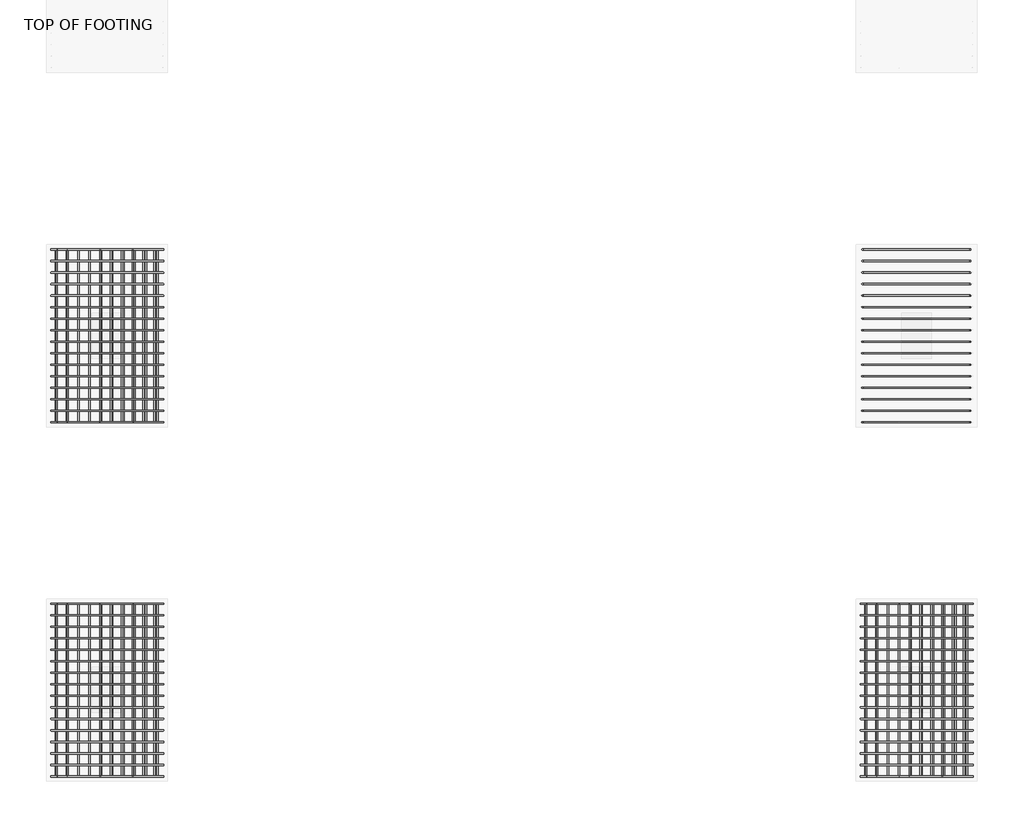
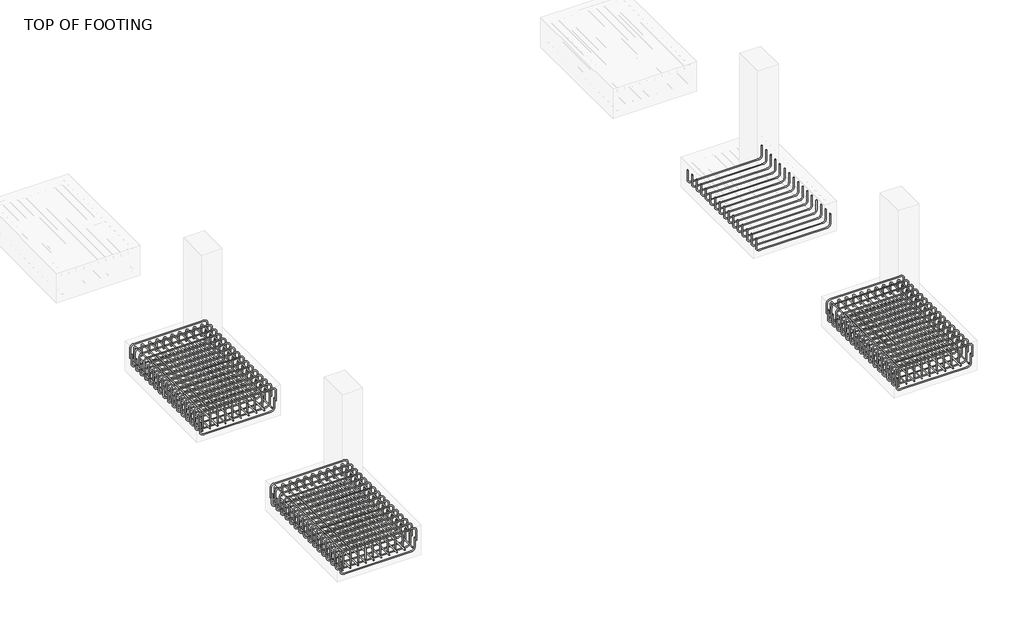
# One storey, part 2 of 8: 13 reinforcing bars.
"""IFC4 building model written with IfcOpenShell, lengths in millimetres."""

from ifc_helpers import new_model, si_unit, point, frame, origin, place, context, project, spatial, polyline, circle_curve, trimmed, segment, composite_curve, source, transform, mapped, element, save
from ifc_brep_helpers import swept_disk

model = new_model("IFC4")

# Units and contexts
model_context = context("Model", 3, world=origin())
ifc_project = project(units=[si_unit("LENGTHUNIT", "METRE", prefix="MILLI")], contexts=[model_context])

# Site, building, storey
site = spatial("IfcSite", under=ifc_project)
building = spatial("IfcBuilding", under=site)
storey = spatial("IfcBuildingStorey", under=building, Name="TOP OF FOOTING", Elevation=-1828.8)

# Reinforcing bars
placement = place(None, origin())
reinforcing_bar_shape = source(origin(), model_context, "Body", "SolidModel", [
    swept_disk(composite_curve([segment(polyline([(-11301.5220197, 6126.3508557, -2021.4413313), (-11301.5220197, 6126.3508557, -2168.7413313)]), True, "CONTINUOUS"), segment(trimmed(circle_curve(frame((-11347.8720197, 6126.3508557, -2168.7413313), z_axis=(0.0, 1.0, 0.0), x_axis=(46.350000000000364, 0.0, 0.0)), 46.35), [point((-11301.5220197, 6126.3508557, -2168.7413313))], [point((-11347.8720197, 6126.3508557, -2215.0913313))], True, "CARTESIAN"), True, "CONTINUOUS"), segment(polyline([(-11347.8720197, 6126.3508557, -2215.0913313), (-12320.167031, 6126.3508557, -2215.0913313)]), True, "CONTINUOUS"), segment(trimmed(circle_curve(frame((-12320.167031, 6126.3508557, -2168.7413313), z_axis=(0.0, 1.0, 0.0), x_axis=(0.0, 0.0, -46.34999999999991)), 46.35), [point((-12320.167031, 6126.3508557, -2215.0913313))], [point((-12366.517031, 6126.3508557, -2168.7413313))], True, "CARTESIAN"), True, "CONTINUOUS"), segment(polyline([(-12366.517031, 6126.3508557, -2168.7413313), (-12366.517031, 6126.3508557, -2021.4413313)]), True, "CONTINUOUS")], self_intersect=False), 6.35),
])
element("IfcReinforcingBar", 1, at=placement, inside=storey, context=model_context, shape_type="MappedRepresentation", body=[
    mapped(reinforcing_bar_shape, transform((0.0, 0.0, 0.0), x_axis=(1.0, 0.0, 0.0), y_axis=(0.0, 1.0, 0.0), z_axis=(0.0, 0.0, 1.0))),
    mapped(reinforcing_bar_shape, transform((0.0, -113.82, 0.0), x_axis=(1.0, 0.0, 0.0), y_axis=(0.0, 1.0, 0.0), z_axis=(0.0, 0.0, 1.0))),
    mapped(reinforcing_bar_shape, transform((0.0, -227.64, 0.0), x_axis=(1.0, 0.0, 0.0), y_axis=(0.0, 1.0, 0.0), z_axis=(0.0, 0.0, 1.0))),
    mapped(reinforcing_bar_shape, transform((0.0, -341.46, 0.0), x_axis=(1.0, 0.0, 0.0), y_axis=(0.0, 1.0, 0.0), z_axis=(0.0, 0.0, 1.0))),
    mapped(reinforcing_bar_shape, transform((0.0, -455.28, 0.0), x_axis=(1.0, 0.0, 0.0), y_axis=(0.0, 1.0, 0.0), z_axis=(0.0, 0.0, 1.0))),
    mapped(reinforcing_bar_shape, transform((0.0, -569.1, 0.0), x_axis=(1.0, 0.0, 0.0), y_axis=(0.0, 1.0, 0.0), z_axis=(0.0, 0.0, 1.0))),
    mapped(reinforcing_bar_shape, transform((0.0, -682.92, 0.0), x_axis=(1.0, 0.0, 0.0), y_axis=(0.0, 1.0, 0.0), z_axis=(0.0, 0.0, 1.0))),
    mapped(reinforcing_bar_shape, transform((0.0, -796.74, 0.0), x_axis=(1.0, 0.0, 0.0), y_axis=(0.0, 1.0, 0.0), z_axis=(0.0, 0.0, 1.0))),
    mapped(reinforcing_bar_shape, transform((0.0, -910.56, 0.0), x_axis=(1.0, 0.0, 0.0), y_axis=(0.0, 1.0, 0.0), z_axis=(0.0, 0.0, 1.0))),
    mapped(reinforcing_bar_shape, transform((0.0, -1024.38, 0.0), x_axis=(1.0, 0.0, 0.0), y_axis=(0.0, 1.0, 0.0), z_axis=(0.0, 0.0, 1.0))),
    mapped(reinforcing_bar_shape, transform((0.0, -1138.2, 0.0), x_axis=(1.0, 0.0, 0.0), y_axis=(0.0, 1.0, 0.0), z_axis=(0.0, 0.0, 1.0))),
    mapped(reinforcing_bar_shape, transform((0.0, -1252.02, 0.0), x_axis=(1.0, 0.0, 0.0), y_axis=(0.0, 1.0, 0.0), z_axis=(0.0, 0.0, 1.0))),
    mapped(reinforcing_bar_shape, transform((0.0, -1365.84, 0.0), x_axis=(1.0, 0.0, 0.0), y_axis=(0.0, 1.0, 0.0), z_axis=(0.0, 0.0, 1.0))),
    mapped(reinforcing_bar_shape, transform((0.0, -1479.66, 0.0), x_axis=(1.0, 0.0, 0.0), y_axis=(0.0, 1.0, 0.0), z_axis=(0.0, 0.0, 1.0))),
    mapped(reinforcing_bar_shape, transform((0.0, -1593.48, 0.0), x_axis=(1.0, 0.0, 0.0), y_axis=(0.0, 1.0, 0.0), z_axis=(0.0, 0.0, 1.0))),
    mapped(reinforcing_bar_shape, transform((0.0, -1707.3, 0.0), x_axis=(1.0, 0.0, 0.0), y_axis=(0.0, 1.0, 0.0), z_axis=(0.0, 0.0, 1.0))),
])
reinforcing_bar_2_shape = source(origin(), model_context, "Body", "SolidModel", [
    swept_disk(composite_curve([segment(polyline([(-12384.3374017, 6126.3508557, -2068.8), (-12384.3374017, 6126.3508557, -1921.5)]), True, "CONTINUOUS"), segment(trimmed(circle_curve(frame((-12337.9874017, 6126.3508557, -1921.5), z_axis=(0.0, 1.0, 0.0), x_axis=(-46.350000000000364, 0.0, 0.0)), 46.35), [point((-12384.3374017, 6126.3508557, -1921.5))], [point((-12337.9874017, 6126.3508557, -1875.15))], True, "CARTESIAN"), True, "CONTINUOUS"), segment(polyline([(-12337.9874017, 6126.3508557, -1875.15), (-11323.3874017, 6126.3508557, -1875.15)]), True, "CONTINUOUS"), segment(trimmed(circle_curve(frame((-11323.3874017, 6126.3508557, -1921.5), z_axis=(0.0, 1.0, 0.0), x_axis=(0.0, 0.0, 46.34999999999991)), 46.35), [point((-11323.3874017, 6126.3508557, -1875.15))], [point((-11277.0374017, 6126.3508557, -1921.5))], True, "CARTESIAN"), True, "CONTINUOUS"), segment(polyline([(-11277.0374017, 6126.3508557, -1921.5), (-11277.0374017, 6126.3508557, -2068.8)]), True, "CONTINUOUS")], self_intersect=False), 6.35),
])
element("IfcReinforcingBar", 2, at=placement, inside=storey, context=model_context, shape_type="MappedRepresentation", body=[
    mapped(reinforcing_bar_2_shape, transform((0.0, 0.0, 0.0), x_axis=(1.0, 0.0, 0.0), y_axis=(0.0, 1.0, 0.0), z_axis=(0.0, 0.0, 1.0))),
    mapped(reinforcing_bar_2_shape, transform((0.0, -113.82, 0.0), x_axis=(1.0, 0.0, 0.0), y_axis=(0.0, 1.0, 0.0), z_axis=(0.0, 0.0, 1.0))),
    mapped(reinforcing_bar_2_shape, transform((0.0, -227.64, 0.0), x_axis=(1.0, 0.0, 0.0), y_axis=(0.0, 1.0, 0.0), z_axis=(0.0, 0.0, 1.0))),
    mapped(reinforcing_bar_2_shape, transform((0.0, -341.46, 0.0), x_axis=(1.0, 0.0, 0.0), y_axis=(0.0, 1.0, 0.0), z_axis=(0.0, 0.0, 1.0))),
    mapped(reinforcing_bar_2_shape, transform((0.0, -455.28, 0.0), x_axis=(1.0, 0.0, 0.0), y_axis=(0.0, 1.0, 0.0), z_axis=(0.0, 0.0, 1.0))),
    mapped(reinforcing_bar_2_shape, transform((0.0, -569.1, 0.0), x_axis=(1.0, 0.0, 0.0), y_axis=(0.0, 1.0, 0.0), z_axis=(0.0, 0.0, 1.0))),
    mapped(reinforcing_bar_2_shape, transform((0.0, -682.92, 0.0), x_axis=(1.0, 0.0, 0.0), y_axis=(0.0, 1.0, 0.0), z_axis=(0.0, 0.0, 1.0))),
    mapped(reinforcing_bar_2_shape, transform((0.0, -796.74, 0.0), x_axis=(1.0, 0.0, 0.0), y_axis=(0.0, 1.0, 0.0), z_axis=(0.0, 0.0, 1.0))),
    mapped(reinforcing_bar_2_shape, transform((0.0, -910.56, 0.0), x_axis=(1.0, 0.0, 0.0), y_axis=(0.0, 1.0, 0.0), z_axis=(0.0, 0.0, 1.0))),
    mapped(reinforcing_bar_2_shape, transform((0.0, -1024.38, 0.0), x_axis=(1.0, 0.0, 0.0), y_axis=(0.0, 1.0, 0.0), z_axis=(0.0, 0.0, 1.0))),
    mapped(reinforcing_bar_2_shape, transform((0.0, -1138.2, 0.0), x_axis=(1.0, 0.0, 0.0), y_axis=(0.0, 1.0, 0.0), z_axis=(0.0, 0.0, 1.0))),
    mapped(reinforcing_bar_2_shape, transform((0.0, -1252.02, 0.0), x_axis=(1.0, 0.0, 0.0), y_axis=(0.0, 1.0, 0.0), z_axis=(0.0, 0.0, 1.0))),
    mapped(reinforcing_bar_2_shape, transform((0.0, -1365.84, 0.0), x_axis=(1.0, 0.0, 0.0), y_axis=(0.0, 1.0, 0.0), z_axis=(0.0, 0.0, 1.0))),
    mapped(reinforcing_bar_2_shape, transform((0.0, -1479.66, 0.0), x_axis=(1.0, 0.0, 0.0), y_axis=(0.0, 1.0, 0.0), z_axis=(0.0, 0.0, 1.0))),
    mapped(reinforcing_bar_2_shape, transform((0.0, -1593.48, 0.0), x_axis=(1.0, 0.0, 0.0), y_axis=(0.0, 1.0, 0.0), z_axis=(0.0, 0.0, 1.0))),
    mapped(reinforcing_bar_2_shape, transform((0.0, -1707.3, 0.0), x_axis=(1.0, 0.0, 0.0), y_axis=(0.0, 1.0, 0.0), z_axis=(0.0, 0.0, 1.0))),
])
reinforcing_bar_3_shape = source(origin(), model_context, "Body", "SolidModel", [
    swept_disk(composite_curve([segment(polyline([(-12339.592709, 6132.7008557, -2155.1176129), (-12339.592709, 4412.7008557, -2155.1176129)]), True, "CONTINUOUS")], self_intersect=False), 6.35),
])
element("IfcReinforcingBar", 3, at=placement, inside=storey, context=model_context, shape_type="MappedRepresentation", body=[
    mapped(reinforcing_bar_3_shape, transform((0.0, 0.0, 0.0), x_axis=(1.0, 0.0, 0.0), y_axis=(0.0, 1.0, 0.0), z_axis=(0.0, 0.0, 1.0))),
    mapped(reinforcing_bar_3_shape, transform((111.602188, 0.0, 0.0), x_axis=(1.0, 0.0, 0.0), y_axis=(0.0, 1.0, 0.0), z_axis=(0.0, 0.0, 1.0))),
    mapped(reinforcing_bar_3_shape, transform((223.2043759, 0.0, 0.0), x_axis=(1.0, 0.0, 0.0), y_axis=(0.0, 1.0, 0.0), z_axis=(0.0, 0.0, 1.0))),
    mapped(reinforcing_bar_3_shape, transform((334.8065639, 0.0, 0.0), x_axis=(1.0, 0.0, 0.0), y_axis=(0.0, 1.0, 0.0), z_axis=(0.0, 0.0, 1.0))),
    mapped(reinforcing_bar_3_shape, transform((446.4087519, 0.0, 0.0), x_axis=(1.0, 0.0, 0.0), y_axis=(0.0, 1.0, 0.0), z_axis=(0.0, 0.0, 1.0))),
    mapped(reinforcing_bar_3_shape, transform((558.0109398, 0.0, 0.0), x_axis=(1.0, 0.0, 0.0), y_axis=(0.0, 1.0, 0.0), z_axis=(0.0, 0.0, 1.0))),
    mapped(reinforcing_bar_3_shape, transform((669.6131278, 0.0, 0.0), x_axis=(1.0, 0.0, 0.0), y_axis=(0.0, 1.0, 0.0), z_axis=(0.0, 0.0, 1.0))),
    mapped(reinforcing_bar_3_shape, transform((781.2153158, 0.0, 0.0), x_axis=(1.0, 0.0, 0.0), y_axis=(0.0, 1.0, 0.0), z_axis=(0.0, 0.0, 1.0))),
    mapped(reinforcing_bar_3_shape, transform((892.8175037, 0.0, 0.0), x_axis=(1.0, 0.0, 0.0), y_axis=(0.0, 1.0, 0.0), z_axis=(0.0, 0.0, 1.0))),
    mapped(reinforcing_bar_3_shape, transform((1004.4196917, 0.0, 0.0), x_axis=(1.0, 0.0, 0.0), y_axis=(0.0, 1.0, 0.0), z_axis=(0.0, 0.0, 1.0))),
])
reinforcing_bar_4_shape = source(origin(), model_context, "Body", "SolidModel", [
    swept_disk(composite_curve([segment(polyline([(-11364.2651981, 6126.3508557, -2094.6521303), (-11364.2651981, 6126.3508557, -1947.3521303)]), True, "CONTINUOUS"), segment(trimmed(circle_curve(frame((-11364.2651981, 6080.0008557, -1947.3521303), z_axis=(1.0, 0.0, 0.0), x_axis=(0.0, 46.349999999999454, 0.0)), 46.35), [point((-11364.2651981, 6126.3508557, -1947.3521303))], [point((-11364.2651981, 6080.0008557, -1901.0021303))], True, "CARTESIAN"), True, "CONTINUOUS"), segment(polyline([(-11364.2651981, 6080.0008557, -1901.0021303), (-11364.2651981, 4465.4008557, -1901.0021303)]), True, "CONTINUOUS"), segment(trimmed(circle_curve(frame((-11364.2651981, 4465.4008557, -1947.3521303), z_axis=(1.0, 0.0, 0.0), x_axis=(0.0, 0.0, 46.34999999999991)), 46.35), [point((-11364.2651981, 4465.4008557, -1901.0021303))], [point((-11364.2651981, 4419.0508557, -1947.3521303))], True, "CARTESIAN"), True, "CONTINUOUS"), segment(polyline([(-11364.2651981, 4419.0508557, -1947.3521303), (-11364.2651981, 4419.0508557, -2094.6521303)]), True, "CONTINUOUS")], self_intersect=False), 6.35),
])
element("IfcReinforcingBar", 4, at=placement, inside=storey, context=model_context, shape_type="MappedRepresentation", body=[
    mapped(reinforcing_bar_4_shape, transform((0.0, 0.0, 0.0), x_axis=(1.0, 0.0, 0.0), y_axis=(0.0, 1.0, 0.0), z_axis=(0.0, 0.0, 1.0))),
    mapped(reinforcing_bar_4_shape, transform((-107.1680233, 0.0, 0.0), x_axis=(1.0, 0.0, 0.0), y_axis=(0.0, 1.0, 0.0), z_axis=(0.0, 0.0, 1.0))),
    mapped(reinforcing_bar_4_shape, transform((-214.3360466, 0.0, 0.0), x_axis=(1.0, 0.0, 0.0), y_axis=(0.0, 1.0, 0.0), z_axis=(0.0, 0.0, 1.0))),
    mapped(reinforcing_bar_4_shape, transform((-321.5040699, 0.0, 0.0), x_axis=(1.0, 0.0, 0.0), y_axis=(0.0, 1.0, 0.0), z_axis=(0.0, 0.0, 1.0))),
    mapped(reinforcing_bar_4_shape, transform((-428.6720932, 0.0, 0.0), x_axis=(1.0, 0.0, 0.0), y_axis=(0.0, 1.0, 0.0), z_axis=(0.0, 0.0, 1.0))),
    mapped(reinforcing_bar_4_shape, transform((-535.8401165, 0.0, 0.0), x_axis=(1.0, 0.0, 0.0), y_axis=(0.0, 1.0, 0.0), z_axis=(0.0, 0.0, 1.0))),
    mapped(reinforcing_bar_4_shape, transform((-643.0081398, 0.0, 0.0), x_axis=(1.0, 0.0, 0.0), y_axis=(0.0, 1.0, 0.0), z_axis=(0.0, 0.0, 1.0))),
    mapped(reinforcing_bar_4_shape, transform((-750.176163, 0.0, 0.0), x_axis=(1.0, 0.0, 0.0), y_axis=(0.0, 1.0, 0.0), z_axis=(0.0, 0.0, 1.0))),
    mapped(reinforcing_bar_4_shape, transform((-857.3441863, 0.0, 0.0), x_axis=(1.0, 0.0, 0.0), y_axis=(0.0, 1.0, 0.0), z_axis=(0.0, 0.0, 1.0))),
    mapped(reinforcing_bar_4_shape, transform((-964.5122096, 0.0, 0.0), x_axis=(1.0, 0.0, 0.0), y_axis=(0.0, 1.0, 0.0), z_axis=(0.0, 0.0, 1.0))),
])
reinforcing_bar_5_shape = source(origin(), model_context, "Body", "SolidModel", [
    swept_disk(composite_curve([segment(polyline([(-11301.5220197, 2626.3508557, -2021.4413313), (-11301.5220197, 2626.3508557, -2168.7413313)]), True, "CONTINUOUS"), segment(trimmed(circle_curve(frame((-11347.8720197, 2626.3508557, -2168.7413313), z_axis=(0.0, 1.0, 0.0), x_axis=(46.350000000000364, 0.0, 0.0)), 46.35), [point((-11301.5220197, 2626.3508557, -2168.7413313))], [point((-11347.8720197, 2626.3508557, -2215.0913313))], True, "CARTESIAN"), True, "CONTINUOUS"), segment(polyline([(-11347.8720197, 2626.3508557, -2215.0913313), (-12320.167031, 2626.3508557, -2215.0913313)]), True, "CONTINUOUS"), segment(trimmed(circle_curve(frame((-12320.167031, 2626.3508557, -2168.7413313), z_axis=(0.0, 1.0, 0.0), x_axis=(0.0, 0.0, -46.34999999999991)), 46.35), [point((-12320.167031, 2626.3508557, -2215.0913313))], [point((-12366.517031, 2626.3508557, -2168.7413313))], True, "CARTESIAN"), True, "CONTINUOUS"), segment(polyline([(-12366.517031, 2626.3508557, -2168.7413313), (-12366.517031, 2626.3508557, -2021.4413313)]), True, "CONTINUOUS")], self_intersect=False), 6.35),
])
element("IfcReinforcingBar", 5, at=placement, inside=storey, context=model_context, shape_type="MappedRepresentation", body=[
    mapped(reinforcing_bar_5_shape, transform((0.0, 0.0, 0.0), x_axis=(1.0, 0.0, 0.0), y_axis=(0.0, 1.0, 0.0), z_axis=(0.0, 0.0, 1.0))),
    mapped(reinforcing_bar_5_shape, transform((0.0, -113.82, 0.0), x_axis=(1.0, 0.0, 0.0), y_axis=(0.0, 1.0, 0.0), z_axis=(0.0, 0.0, 1.0))),
    mapped(reinforcing_bar_5_shape, transform((0.0, -227.64, 0.0), x_axis=(1.0, 0.0, 0.0), y_axis=(0.0, 1.0, 0.0), z_axis=(0.0, 0.0, 1.0))),
    mapped(reinforcing_bar_5_shape, transform((0.0, -341.46, 0.0), x_axis=(1.0, 0.0, 0.0), y_axis=(0.0, 1.0, 0.0), z_axis=(0.0, 0.0, 1.0))),
    mapped(reinforcing_bar_5_shape, transform((0.0, -455.28, 0.0), x_axis=(1.0, 0.0, 0.0), y_axis=(0.0, 1.0, 0.0), z_axis=(0.0, 0.0, 1.0))),
    mapped(reinforcing_bar_5_shape, transform((0.0, -569.1, 0.0), x_axis=(1.0, 0.0, 0.0), y_axis=(0.0, 1.0, 0.0), z_axis=(0.0, 0.0, 1.0))),
    mapped(reinforcing_bar_5_shape, transform((0.0, -682.92, 0.0), x_axis=(1.0, 0.0, 0.0), y_axis=(0.0, 1.0, 0.0), z_axis=(0.0, 0.0, 1.0))),
    mapped(reinforcing_bar_5_shape, transform((0.0, -796.74, 0.0), x_axis=(1.0, 0.0, 0.0), y_axis=(0.0, 1.0, 0.0), z_axis=(0.0, 0.0, 1.0))),
    mapped(reinforcing_bar_5_shape, transform((0.0, -910.56, 0.0), x_axis=(1.0, 0.0, 0.0), y_axis=(0.0, 1.0, 0.0), z_axis=(0.0, 0.0, 1.0))),
    mapped(reinforcing_bar_5_shape, transform((0.0, -1024.38, 0.0), x_axis=(1.0, 0.0, 0.0), y_axis=(0.0, 1.0, 0.0), z_axis=(0.0, 0.0, 1.0))),
    mapped(reinforcing_bar_5_shape, transform((0.0, -1138.2, 0.0), x_axis=(1.0, 0.0, 0.0), y_axis=(0.0, 1.0, 0.0), z_axis=(0.0, 0.0, 1.0))),
    mapped(reinforcing_bar_5_shape, transform((0.0, -1252.02, 0.0), x_axis=(1.0, 0.0, 0.0), y_axis=(0.0, 1.0, 0.0), z_axis=(0.0, 0.0, 1.0))),
    mapped(reinforcing_bar_5_shape, transform((0.0, -1365.84, 0.0), x_axis=(1.0, 0.0, 0.0), y_axis=(0.0, 1.0, 0.0), z_axis=(0.0, 0.0, 1.0))),
    mapped(reinforcing_bar_5_shape, transform((0.0, -1479.66, 0.0), x_axis=(1.0, 0.0, 0.0), y_axis=(0.0, 1.0, 0.0), z_axis=(0.0, 0.0, 1.0))),
    mapped(reinforcing_bar_5_shape, transform((0.0, -1593.48, 0.0), x_axis=(1.0, 0.0, 0.0), y_axis=(0.0, 1.0, 0.0), z_axis=(0.0, 0.0, 1.0))),
    mapped(reinforcing_bar_5_shape, transform((0.0, -1707.3, 0.0), x_axis=(1.0, 0.0, 0.0), y_axis=(0.0, 1.0, 0.0), z_axis=(0.0, 0.0, 1.0))),
])
reinforcing_bar_6_shape = source(origin(), model_context, "Body", "SolidModel", [
    swept_disk(composite_curve([segment(polyline([(-12384.3374017, 2626.3508557, -2068.8), (-12384.3374017, 2626.3508557, -1921.5)]), True, "CONTINUOUS"), segment(trimmed(circle_curve(frame((-12337.9874017, 2626.3508557, -1921.5), z_axis=(0.0, 1.0, 0.0), x_axis=(-46.350000000000364, 0.0, 0.0)), 46.35), [point((-12384.3374017, 2626.3508557, -1921.5))], [point((-12337.9874017, 2626.3508557, -1875.15))], True, "CARTESIAN"), True, "CONTINUOUS"), segment(polyline([(-12337.9874017, 2626.3508557, -1875.15), (-11323.3874017, 2626.3508557, -1875.15)]), True, "CONTINUOUS"), segment(trimmed(circle_curve(frame((-11323.3874017, 2626.3508557, -1921.5), z_axis=(0.0, 1.0, 0.0), x_axis=(0.0, 0.0, 46.34999999999991)), 46.35), [point((-11323.3874017, 2626.3508557, -1875.15))], [point((-11277.0374017, 2626.3508557, -1921.5))], True, "CARTESIAN"), True, "CONTINUOUS"), segment(polyline([(-11277.0374017, 2626.3508557, -1921.5), (-11277.0374017, 2626.3508557, -2068.8)]), True, "CONTINUOUS")], self_intersect=False), 6.35),
])
element("IfcReinforcingBar", 6, at=placement, inside=storey, context=model_context, shape_type="MappedRepresentation", body=[
    mapped(reinforcing_bar_6_shape, transform((0.0, 0.0, 0.0), x_axis=(1.0, 0.0, 0.0), y_axis=(0.0, 1.0, 0.0), z_axis=(0.0, 0.0, 1.0))),
    mapped(reinforcing_bar_6_shape, transform((0.0, -113.82, 0.0), x_axis=(1.0, 0.0, 0.0), y_axis=(0.0, 1.0, 0.0), z_axis=(0.0, 0.0, 1.0))),
    mapped(reinforcing_bar_6_shape, transform((0.0, -227.64, 0.0), x_axis=(1.0, 0.0, 0.0), y_axis=(0.0, 1.0, 0.0), z_axis=(0.0, 0.0, 1.0))),
    mapped(reinforcing_bar_6_shape, transform((0.0, -341.46, 0.0), x_axis=(1.0, 0.0, 0.0), y_axis=(0.0, 1.0, 0.0), z_axis=(0.0, 0.0, 1.0))),
    mapped(reinforcing_bar_6_shape, transform((0.0, -455.28, 0.0), x_axis=(1.0, 0.0, 0.0), y_axis=(0.0, 1.0, 0.0), z_axis=(0.0, 0.0, 1.0))),
    mapped(reinforcing_bar_6_shape, transform((0.0, -569.1, 0.0), x_axis=(1.0, 0.0, 0.0), y_axis=(0.0, 1.0, 0.0), z_axis=(0.0, 0.0, 1.0))),
    mapped(reinforcing_bar_6_shape, transform((0.0, -682.92, 0.0), x_axis=(1.0, 0.0, 0.0), y_axis=(0.0, 1.0, 0.0), z_axis=(0.0, 0.0, 1.0))),
    mapped(reinforcing_bar_6_shape, transform((0.0, -796.74, 0.0), x_axis=(1.0, 0.0, 0.0), y_axis=(0.0, 1.0, 0.0), z_axis=(0.0, 0.0, 1.0))),
    mapped(reinforcing_bar_6_shape, transform((0.0, -910.56, 0.0), x_axis=(1.0, 0.0, 0.0), y_axis=(0.0, 1.0, 0.0), z_axis=(0.0, 0.0, 1.0))),
    mapped(reinforcing_bar_6_shape, transform((0.0, -1024.38, 0.0), x_axis=(1.0, 0.0, 0.0), y_axis=(0.0, 1.0, 0.0), z_axis=(0.0, 0.0, 1.0))),
    mapped(reinforcing_bar_6_shape, transform((0.0, -1138.2, 0.0), x_axis=(1.0, 0.0, 0.0), y_axis=(0.0, 1.0, 0.0), z_axis=(0.0, 0.0, 1.0))),
    mapped(reinforcing_bar_6_shape, transform((0.0, -1252.02, 0.0), x_axis=(1.0, 0.0, 0.0), y_axis=(0.0, 1.0, 0.0), z_axis=(0.0, 0.0, 1.0))),
    mapped(reinforcing_bar_6_shape, transform((0.0, -1365.84, 0.0), x_axis=(1.0, 0.0, 0.0), y_axis=(0.0, 1.0, 0.0), z_axis=(0.0, 0.0, 1.0))),
    mapped(reinforcing_bar_6_shape, transform((0.0, -1479.66, 0.0), x_axis=(1.0, 0.0, 0.0), y_axis=(0.0, 1.0, 0.0), z_axis=(0.0, 0.0, 1.0))),
    mapped(reinforcing_bar_6_shape, transform((0.0, -1593.48, 0.0), x_axis=(1.0, 0.0, 0.0), y_axis=(0.0, 1.0, 0.0), z_axis=(0.0, 0.0, 1.0))),
    mapped(reinforcing_bar_6_shape, transform((0.0, -1707.3, 0.0), x_axis=(1.0, 0.0, 0.0), y_axis=(0.0, 1.0, 0.0), z_axis=(0.0, 0.0, 1.0))),
])
reinforcing_bar_7_shape = source(origin(), model_context, "Body", "SolidModel", [
    swept_disk(composite_curve([segment(polyline([(-12339.592709, 2632.7008557, -2155.1176129), (-12339.592709, 912.7008557, -2155.1176129)]), True, "CONTINUOUS")], self_intersect=False), 6.35),
])
element("IfcReinforcingBar", 7, at=placement, inside=storey, context=model_context, shape_type="MappedRepresentation", body=[
    mapped(reinforcing_bar_7_shape, transform((0.0, 0.0, 0.0), x_axis=(1.0, 0.0, 0.0), y_axis=(0.0, 1.0, 0.0), z_axis=(0.0, 0.0, 1.0))),
    mapped(reinforcing_bar_7_shape, transform((111.602188, 0.0, 0.0), x_axis=(1.0, 0.0, 0.0), y_axis=(0.0, 1.0, 0.0), z_axis=(0.0, 0.0, 1.0))),
    mapped(reinforcing_bar_7_shape, transform((223.2043759, 0.0, 0.0), x_axis=(1.0, 0.0, 0.0), y_axis=(0.0, 1.0, 0.0), z_axis=(0.0, 0.0, 1.0))),
    mapped(reinforcing_bar_7_shape, transform((334.8065639, 0.0, 0.0), x_axis=(1.0, 0.0, 0.0), y_axis=(0.0, 1.0, 0.0), z_axis=(0.0, 0.0, 1.0))),
    mapped(reinforcing_bar_7_shape, transform((446.4087519, 0.0, 0.0), x_axis=(1.0, 0.0, 0.0), y_axis=(0.0, 1.0, 0.0), z_axis=(0.0, 0.0, 1.0))),
    mapped(reinforcing_bar_7_shape, transform((558.0109398, 0.0, 0.0), x_axis=(1.0, 0.0, 0.0), y_axis=(0.0, 1.0, 0.0), z_axis=(0.0, 0.0, 1.0))),
    mapped(reinforcing_bar_7_shape, transform((669.6131278, 0.0, 0.0), x_axis=(1.0, 0.0, 0.0), y_axis=(0.0, 1.0, 0.0), z_axis=(0.0, 0.0, 1.0))),
    mapped(reinforcing_bar_7_shape, transform((781.2153158, 0.0, 0.0), x_axis=(1.0, 0.0, 0.0), y_axis=(0.0, 1.0, 0.0), z_axis=(0.0, 0.0, 1.0))),
    mapped(reinforcing_bar_7_shape, transform((892.8175037, 0.0, 0.0), x_axis=(1.0, 0.0, 0.0), y_axis=(0.0, 1.0, 0.0), z_axis=(0.0, 0.0, 1.0))),
    mapped(reinforcing_bar_7_shape, transform((1004.4196917, 0.0, 0.0), x_axis=(1.0, 0.0, 0.0), y_axis=(0.0, 1.0, 0.0), z_axis=(0.0, 0.0, 1.0))),
])
reinforcing_bar_8_shape = source(origin(), model_context, "Body", "SolidModel", [
    swept_disk(composite_curve([segment(polyline([(-11364.2651981, 2626.3508557, -2094.6521303), (-11364.2651981, 2626.3508557, -1947.3521303)]), True, "CONTINUOUS"), segment(trimmed(circle_curve(frame((-11364.2651981, 2580.0008557, -1947.3521303), z_axis=(1.0, 0.0, 0.0), x_axis=(0.0, 46.34999999999991, 0.0)), 46.35), [point((-11364.2651981, 2626.3508557, -1947.3521303))], [point((-11364.2651981, 2580.0008557, -1901.0021303))], True, "CARTESIAN"), True, "CONTINUOUS"), segment(polyline([(-11364.2651981, 2580.0008557, -1901.0021303), (-11364.2651981, 965.4008557, -1901.0021303)]), True, "CONTINUOUS"), segment(trimmed(circle_curve(frame((-11364.2651981, 965.4008557, -1947.3521303), z_axis=(1.0, 0.0, 0.0), x_axis=(0.0, 0.0, 46.34999999999991)), 46.35), [point((-11364.2651981, 965.4008557, -1901.0021303))], [point((-11364.2651981, 919.0508557, -1947.3521303))], True, "CARTESIAN"), True, "CONTINUOUS"), segment(polyline([(-11364.2651981, 919.0508557, -1947.3521303), (-11364.2651981, 919.0508557, -2094.6521303)]), True, "CONTINUOUS")], self_intersect=False), 6.35),
])
element("IfcReinforcingBar", 8, at=placement, inside=storey, context=model_context, shape_type="MappedRepresentation", body=[
    mapped(reinforcing_bar_8_shape, transform((0.0, 0.0, 0.0), x_axis=(1.0, 0.0, 0.0), y_axis=(0.0, 1.0, 0.0), z_axis=(0.0, 0.0, 1.0))),
    mapped(reinforcing_bar_8_shape, transform((-107.1680233, 0.0, 0.0), x_axis=(1.0, 0.0, 0.0), y_axis=(0.0, 1.0, 0.0), z_axis=(0.0, 0.0, 1.0))),
    mapped(reinforcing_bar_8_shape, transform((-214.3360466, 0.0, 0.0), x_axis=(1.0, 0.0, 0.0), y_axis=(0.0, 1.0, 0.0), z_axis=(0.0, 0.0, 1.0))),
    mapped(reinforcing_bar_8_shape, transform((-321.5040699, 0.0, 0.0), x_axis=(1.0, 0.0, 0.0), y_axis=(0.0, 1.0, 0.0), z_axis=(0.0, 0.0, 1.0))),
    mapped(reinforcing_bar_8_shape, transform((-428.6720932, 0.0, 0.0), x_axis=(1.0, 0.0, 0.0), y_axis=(0.0, 1.0, 0.0), z_axis=(0.0, 0.0, 1.0))),
    mapped(reinforcing_bar_8_shape, transform((-535.8401165, 0.0, 0.0), x_axis=(1.0, 0.0, 0.0), y_axis=(0.0, 1.0, 0.0), z_axis=(0.0, 0.0, 1.0))),
    mapped(reinforcing_bar_8_shape, transform((-643.0081398, 0.0, 0.0), x_axis=(1.0, 0.0, 0.0), y_axis=(0.0, 1.0, 0.0), z_axis=(0.0, 0.0, 1.0))),
    mapped(reinforcing_bar_8_shape, transform((-750.176163, 0.0, 0.0), x_axis=(1.0, 0.0, 0.0), y_axis=(0.0, 1.0, 0.0), z_axis=(0.0, 0.0, 1.0))),
    mapped(reinforcing_bar_8_shape, transform((-857.3441863, 0.0, 0.0), x_axis=(1.0, 0.0, 0.0), y_axis=(0.0, 1.0, 0.0), z_axis=(0.0, 0.0, 1.0))),
    mapped(reinforcing_bar_8_shape, transform((-964.5122096, 0.0, 0.0), x_axis=(1.0, 0.0, 0.0), y_axis=(0.0, 1.0, 0.0), z_axis=(0.0, 0.0, 1.0))),
])
reinforcing_bar_9_shape = source(origin(), model_context, "Body", "SolidModel", [
    swept_disk(composite_curve([segment(polyline([(-3301.5220197, 6126.3508557, -2021.4413313), (-3301.5220197, 6126.3508557, -2168.7413313)]), True, "CONTINUOUS"), segment(trimmed(circle_curve(frame((-3347.8720197, 6126.3508557, -2168.7413313), z_axis=(0.0, 1.0, 0.0), x_axis=(46.34999999999991, 0.0, 0.0)), 46.35), [point((-3301.5220197, 6126.3508557, -2168.7413313))], [point((-3347.8720197, 6126.3508557, -2215.0913313))], True, "CARTESIAN"), True, "CONTINUOUS"), segment(polyline([(-3347.8720197, 6126.3508557, -2215.0913313), (-4320.167031, 6126.3508557, -2215.0913313)]), True, "CONTINUOUS"), segment(trimmed(circle_curve(frame((-4320.167031, 6126.3508557, -2168.7413313), z_axis=(0.0, 1.0, 0.0), x_axis=(0.0, 0.0, -46.34999999999991)), 46.35), [point((-4320.167031, 6126.3508557, -2215.0913313))], [point((-4366.517031, 6126.3508557, -2168.7413313))], True, "CARTESIAN"), True, "CONTINUOUS"), segment(polyline([(-4366.517031, 6126.3508557, -2168.7413313), (-4366.517031, 6126.3508557, -2021.4413313)]), True, "CONTINUOUS")], self_intersect=False), 6.35),
])
element("IfcReinforcingBar", 9, at=placement, inside=storey, context=model_context, shape_type="MappedRepresentation", body=[
    mapped(reinforcing_bar_9_shape, transform((0.0, 0.0, 0.0), x_axis=(1.0, 0.0, 0.0), y_axis=(0.0, 1.0, 0.0), z_axis=(0.0, 0.0, 1.0))),
    mapped(reinforcing_bar_9_shape, transform((0.0, -113.82, 0.0), x_axis=(1.0, 0.0, 0.0), y_axis=(0.0, 1.0, 0.0), z_axis=(0.0, 0.0, 1.0))),
    mapped(reinforcing_bar_9_shape, transform((0.0, -227.64, 0.0), x_axis=(1.0, 0.0, 0.0), y_axis=(0.0, 1.0, 0.0), z_axis=(0.0, 0.0, 1.0))),
    mapped(reinforcing_bar_9_shape, transform((0.0, -341.46, 0.0), x_axis=(1.0, 0.0, 0.0), y_axis=(0.0, 1.0, 0.0), z_axis=(0.0, 0.0, 1.0))),
    mapped(reinforcing_bar_9_shape, transform((0.0, -455.28, 0.0), x_axis=(1.0, 0.0, 0.0), y_axis=(0.0, 1.0, 0.0), z_axis=(0.0, 0.0, 1.0))),
    mapped(reinforcing_bar_9_shape, transform((0.0, -569.1, 0.0), x_axis=(1.0, 0.0, 0.0), y_axis=(0.0, 1.0, 0.0), z_axis=(0.0, 0.0, 1.0))),
    mapped(reinforcing_bar_9_shape, transform((0.0, -682.92, 0.0), x_axis=(1.0, 0.0, 0.0), y_axis=(0.0, 1.0, 0.0), z_axis=(0.0, 0.0, 1.0))),
    mapped(reinforcing_bar_9_shape, transform((0.0, -796.74, 0.0), x_axis=(1.0, 0.0, 0.0), y_axis=(0.0, 1.0, 0.0), z_axis=(0.0, 0.0, 1.0))),
    mapped(reinforcing_bar_9_shape, transform((0.0, -910.56, 0.0), x_axis=(1.0, 0.0, 0.0), y_axis=(0.0, 1.0, 0.0), z_axis=(0.0, 0.0, 1.0))),
    mapped(reinforcing_bar_9_shape, transform((0.0, -1024.38, 0.0), x_axis=(1.0, 0.0, 0.0), y_axis=(0.0, 1.0, 0.0), z_axis=(0.0, 0.0, 1.0))),
    mapped(reinforcing_bar_9_shape, transform((0.0, -1138.2, 0.0), x_axis=(1.0, 0.0, 0.0), y_axis=(0.0, 1.0, 0.0), z_axis=(0.0, 0.0, 1.0))),
    mapped(reinforcing_bar_9_shape, transform((0.0, -1252.02, 0.0), x_axis=(1.0, 0.0, 0.0), y_axis=(0.0, 1.0, 0.0), z_axis=(0.0, 0.0, 1.0))),
    mapped(reinforcing_bar_9_shape, transform((0.0, -1365.84, 0.0), x_axis=(1.0, 0.0, 0.0), y_axis=(0.0, 1.0, 0.0), z_axis=(0.0, 0.0, 1.0))),
    mapped(reinforcing_bar_9_shape, transform((0.0, -1479.66, 0.0), x_axis=(1.0, 0.0, 0.0), y_axis=(0.0, 1.0, 0.0), z_axis=(0.0, 0.0, 1.0))),
    mapped(reinforcing_bar_9_shape, transform((0.0, -1593.48, 0.0), x_axis=(1.0, 0.0, 0.0), y_axis=(0.0, 1.0, 0.0), z_axis=(0.0, 0.0, 1.0))),
    mapped(reinforcing_bar_9_shape, transform((0.0, -1707.3, 0.0), x_axis=(1.0, 0.0, 0.0), y_axis=(0.0, 1.0, 0.0), z_axis=(0.0, 0.0, 1.0))),
])
reinforcing_bar_10_shape = source(origin(), model_context, "Body", "SolidModel", [
    swept_disk(composite_curve([segment(polyline([(-3301.5220197, 2626.3508557, -2021.4413313), (-3301.5220197, 2626.3508557, -2168.7413313)]), True, "CONTINUOUS"), segment(trimmed(circle_curve(frame((-3347.8720197, 2626.3508557, -2168.7413313), z_axis=(0.0, 1.0, 0.0), x_axis=(46.34999999999991, 0.0, 0.0)), 46.35), [point((-3301.5220197, 2626.3508557, -2168.7413313))], [point((-3347.8720197, 2626.3508557, -2215.0913313))], True, "CARTESIAN"), True, "CONTINUOUS"), segment(polyline([(-3347.8720197, 2626.3508557, -2215.0913313), (-4320.167031, 2626.3508557, -2215.0913313)]), True, "CONTINUOUS"), segment(trimmed(circle_curve(frame((-4320.167031, 2626.3508557, -2168.7413313), z_axis=(0.0, 1.0, 0.0), x_axis=(0.0, 0.0, -46.34999999999991)), 46.35), [point((-4320.167031, 2626.3508557, -2215.0913313))], [point((-4366.517031, 2626.3508557, -2168.7413313))], True, "CARTESIAN"), True, "CONTINUOUS"), segment(polyline([(-4366.517031, 2626.3508557, -2168.7413313), (-4366.517031, 2626.3508557, -2021.4413313)]), True, "CONTINUOUS")], self_intersect=False), 6.35),
])
element("IfcReinforcingBar", 10, at=placement, inside=storey, context=model_context, shape_type="MappedRepresentation", body=[
    mapped(reinforcing_bar_10_shape, transform((0.0, 0.0, 0.0), x_axis=(1.0, 0.0, 0.0), y_axis=(0.0, 1.0, 0.0), z_axis=(0.0, 0.0, 1.0))),
    mapped(reinforcing_bar_10_shape, transform((0.0, -113.82, 0.0), x_axis=(1.0, 0.0, 0.0), y_axis=(0.0, 1.0, 0.0), z_axis=(0.0, 0.0, 1.0))),
    mapped(reinforcing_bar_10_shape, transform((0.0, -227.64, 0.0), x_axis=(1.0, 0.0, 0.0), y_axis=(0.0, 1.0, 0.0), z_axis=(0.0, 0.0, 1.0))),
    mapped(reinforcing_bar_10_shape, transform((0.0, -341.46, 0.0), x_axis=(1.0, 0.0, 0.0), y_axis=(0.0, 1.0, 0.0), z_axis=(0.0, 0.0, 1.0))),
    mapped(reinforcing_bar_10_shape, transform((0.0, -455.28, 0.0), x_axis=(1.0, 0.0, 0.0), y_axis=(0.0, 1.0, 0.0), z_axis=(0.0, 0.0, 1.0))),
    mapped(reinforcing_bar_10_shape, transform((0.0, -569.1, 0.0), x_axis=(1.0, 0.0, 0.0), y_axis=(0.0, 1.0, 0.0), z_axis=(0.0, 0.0, 1.0))),
    mapped(reinforcing_bar_10_shape, transform((0.0, -682.92, 0.0), x_axis=(1.0, 0.0, 0.0), y_axis=(0.0, 1.0, 0.0), z_axis=(0.0, 0.0, 1.0))),
    mapped(reinforcing_bar_10_shape, transform((0.0, -796.74, 0.0), x_axis=(1.0, 0.0, 0.0), y_axis=(0.0, 1.0, 0.0), z_axis=(0.0, 0.0, 1.0))),
    mapped(reinforcing_bar_10_shape, transform((0.0, -910.56, 0.0), x_axis=(1.0, 0.0, 0.0), y_axis=(0.0, 1.0, 0.0), z_axis=(0.0, 0.0, 1.0))),
    mapped(reinforcing_bar_10_shape, transform((0.0, -1024.38, 0.0), x_axis=(1.0, 0.0, 0.0), y_axis=(0.0, 1.0, 0.0), z_axis=(0.0, 0.0, 1.0))),
    mapped(reinforcing_bar_10_shape, transform((0.0, -1138.2, 0.0), x_axis=(1.0, 0.0, 0.0), y_axis=(0.0, 1.0, 0.0), z_axis=(0.0, 0.0, 1.0))),
    mapped(reinforcing_bar_10_shape, transform((0.0, -1252.02, 0.0), x_axis=(1.0, 0.0, 0.0), y_axis=(0.0, 1.0, 0.0), z_axis=(0.0, 0.0, 1.0))),
    mapped(reinforcing_bar_10_shape, transform((0.0, -1365.84, 0.0), x_axis=(1.0, 0.0, 0.0), y_axis=(0.0, 1.0, 0.0), z_axis=(0.0, 0.0, 1.0))),
    mapped(reinforcing_bar_10_shape, transform((0.0, -1479.66, 0.0), x_axis=(1.0, 0.0, 0.0), y_axis=(0.0, 1.0, 0.0), z_axis=(0.0, 0.0, 1.0))),
    mapped(reinforcing_bar_10_shape, transform((0.0, -1593.48, 0.0), x_axis=(1.0, 0.0, 0.0), y_axis=(0.0, 1.0, 0.0), z_axis=(0.0, 0.0, 1.0))),
    mapped(reinforcing_bar_10_shape, transform((0.0, -1707.3, 0.0), x_axis=(1.0, 0.0, 0.0), y_axis=(0.0, 1.0, 0.0), z_axis=(0.0, 0.0, 1.0))),
])
reinforcing_bar_11_shape = source(origin(), model_context, "Body", "SolidModel", [
    swept_disk(composite_curve([segment(polyline([(-4384.3374017, 2626.3508557, -2068.8), (-4384.3374017, 2626.3508557, -1921.5)]), True, "CONTINUOUS"), segment(trimmed(circle_curve(frame((-4337.9874017, 2626.3508557, -1921.5), z_axis=(0.0, 1.0, 0.0), x_axis=(-46.349999999999454, 0.0, 0.0)), 46.35), [point((-4384.3374017, 2626.3508557, -1921.5))], [point((-4337.9874017, 2626.3508557, -1875.15))], True, "CARTESIAN"), True, "CONTINUOUS"), segment(polyline([(-4337.9874017, 2626.3508557, -1875.15), (-3323.3874017, 2626.3508557, -1875.15)]), True, "CONTINUOUS"), segment(trimmed(circle_curve(frame((-3323.3874017, 2626.3508557, -1921.5), z_axis=(0.0, 1.0, 0.0), x_axis=(0.0, 0.0, 46.34999999999991)), 46.35), [point((-3323.3874017, 2626.3508557, -1875.15))], [point((-3277.0374017, 2626.3508557, -1921.5))], True, "CARTESIAN"), True, "CONTINUOUS"), segment(polyline([(-3277.0374017, 2626.3508557, -1921.5), (-3277.0374017, 2626.3508557, -2068.8)]), True, "CONTINUOUS")], self_intersect=False), 6.35),
])
element("IfcReinforcingBar", 11, at=placement, inside=storey, context=model_context, shape_type="MappedRepresentation", body=[
    mapped(reinforcing_bar_11_shape, transform((0.0, 0.0, 0.0), x_axis=(1.0, 0.0, 0.0), y_axis=(0.0, 1.0, 0.0), z_axis=(0.0, 0.0, 1.0))),
    mapped(reinforcing_bar_11_shape, transform((0.0, -113.82, 0.0), x_axis=(1.0, 0.0, 0.0), y_axis=(0.0, 1.0, 0.0), z_axis=(0.0, 0.0, 1.0))),
    mapped(reinforcing_bar_11_shape, transform((0.0, -227.64, 0.0), x_axis=(1.0, 0.0, 0.0), y_axis=(0.0, 1.0, 0.0), z_axis=(0.0, 0.0, 1.0))),
    mapped(reinforcing_bar_11_shape, transform((0.0, -341.46, 0.0), x_axis=(1.0, 0.0, 0.0), y_axis=(0.0, 1.0, 0.0), z_axis=(0.0, 0.0, 1.0))),
    mapped(reinforcing_bar_11_shape, transform((0.0, -455.28, 0.0), x_axis=(1.0, 0.0, 0.0), y_axis=(0.0, 1.0, 0.0), z_axis=(0.0, 0.0, 1.0))),
    mapped(reinforcing_bar_11_shape, transform((0.0, -569.1, 0.0), x_axis=(1.0, 0.0, 0.0), y_axis=(0.0, 1.0, 0.0), z_axis=(0.0, 0.0, 1.0))),
    mapped(reinforcing_bar_11_shape, transform((0.0, -682.92, 0.0), x_axis=(1.0, 0.0, 0.0), y_axis=(0.0, 1.0, 0.0), z_axis=(0.0, 0.0, 1.0))),
    mapped(reinforcing_bar_11_shape, transform((0.0, -796.74, 0.0), x_axis=(1.0, 0.0, 0.0), y_axis=(0.0, 1.0, 0.0), z_axis=(0.0, 0.0, 1.0))),
    mapped(reinforcing_bar_11_shape, transform((0.0, -910.56, 0.0), x_axis=(1.0, 0.0, 0.0), y_axis=(0.0, 1.0, 0.0), z_axis=(0.0, 0.0, 1.0))),
    mapped(reinforcing_bar_11_shape, transform((0.0, -1024.38, 0.0), x_axis=(1.0, 0.0, 0.0), y_axis=(0.0, 1.0, 0.0), z_axis=(0.0, 0.0, 1.0))),
    mapped(reinforcing_bar_11_shape, transform((0.0, -1138.2, 0.0), x_axis=(1.0, 0.0, 0.0), y_axis=(0.0, 1.0, 0.0), z_axis=(0.0, 0.0, 1.0))),
    mapped(reinforcing_bar_11_shape, transform((0.0, -1252.02, 0.0), x_axis=(1.0, 0.0, 0.0), y_axis=(0.0, 1.0, 0.0), z_axis=(0.0, 0.0, 1.0))),
    mapped(reinforcing_bar_11_shape, transform((0.0, -1365.84, 0.0), x_axis=(1.0, 0.0, 0.0), y_axis=(0.0, 1.0, 0.0), z_axis=(0.0, 0.0, 1.0))),
    mapped(reinforcing_bar_11_shape, transform((0.0, -1479.66, 0.0), x_axis=(1.0, 0.0, 0.0), y_axis=(0.0, 1.0, 0.0), z_axis=(0.0, 0.0, 1.0))),
    mapped(reinforcing_bar_11_shape, transform((0.0, -1593.48, 0.0), x_axis=(1.0, 0.0, 0.0), y_axis=(0.0, 1.0, 0.0), z_axis=(0.0, 0.0, 1.0))),
    mapped(reinforcing_bar_11_shape, transform((0.0, -1707.3, 0.0), x_axis=(1.0, 0.0, 0.0), y_axis=(0.0, 1.0, 0.0), z_axis=(0.0, 0.0, 1.0))),
])
reinforcing_bar_12_shape = source(origin(), model_context, "Body", "SolidModel", [
    swept_disk(composite_curve([segment(polyline([(-4339.592709, 2632.7008557, -2155.1176129), (-4339.592709, 912.7008557, -2155.1176129)]), True, "CONTINUOUS")], self_intersect=False), 6.35),
])
element("IfcReinforcingBar", 12, at=placement, inside=storey, context=model_context, shape_type="MappedRepresentation", body=[
    mapped(reinforcing_bar_12_shape, transform((0.0, 0.0, 0.0), x_axis=(1.0, 0.0, 0.0), y_axis=(0.0, 1.0, 0.0), z_axis=(0.0, 0.0, 1.0))),
    mapped(reinforcing_bar_12_shape, transform((111.602188, 0.0, 0.0), x_axis=(1.0, 0.0, 0.0), y_axis=(0.0, 1.0, 0.0), z_axis=(0.0, 0.0, 1.0))),
    mapped(reinforcing_bar_12_shape, transform((223.2043759, 0.0, 0.0), x_axis=(1.0, 0.0, 0.0), y_axis=(0.0, 1.0, 0.0), z_axis=(0.0, 0.0, 1.0))),
    mapped(reinforcing_bar_12_shape, transform((334.8065639, 0.0, 0.0), x_axis=(1.0, 0.0, 0.0), y_axis=(0.0, 1.0, 0.0), z_axis=(0.0, 0.0, 1.0))),
    mapped(reinforcing_bar_12_shape, transform((446.4087519, 0.0, 0.0), x_axis=(1.0, 0.0, 0.0), y_axis=(0.0, 1.0, 0.0), z_axis=(0.0, 0.0, 1.0))),
    mapped(reinforcing_bar_12_shape, transform((558.0109398, 0.0, 0.0), x_axis=(1.0, 0.0, 0.0), y_axis=(0.0, 1.0, 0.0), z_axis=(0.0, 0.0, 1.0))),
    mapped(reinforcing_bar_12_shape, transform((669.6131278, 0.0, 0.0), x_axis=(1.0, 0.0, 0.0), y_axis=(0.0, 1.0, 0.0), z_axis=(0.0, 0.0, 1.0))),
    mapped(reinforcing_bar_12_shape, transform((781.2153158, 0.0, 0.0), x_axis=(1.0, 0.0, 0.0), y_axis=(0.0, 1.0, 0.0), z_axis=(0.0, 0.0, 1.0))),
    mapped(reinforcing_bar_12_shape, transform((892.8175037, 0.0, 0.0), x_axis=(1.0, 0.0, 0.0), y_axis=(0.0, 1.0, 0.0), z_axis=(0.0, 0.0, 1.0))),
    mapped(reinforcing_bar_12_shape, transform((1004.4196917, 0.0, 0.0), x_axis=(1.0, 0.0, 0.0), y_axis=(0.0, 1.0, 0.0), z_axis=(0.0, 0.0, 1.0))),
])
reinforcing_bar_13_shape = source(origin(), model_context, "Body", "SolidModel", [
    swept_disk(composite_curve([segment(polyline([(-3364.2651981, 2626.3508557, -2094.6521303), (-3364.2651981, 2626.3508557, -1947.3521303)]), True, "CONTINUOUS"), segment(trimmed(circle_curve(frame((-3364.2651981, 2580.0008557, -1947.3521303), z_axis=(1.0, 0.0, 0.0), x_axis=(0.0, 46.34999999999991, 0.0)), 46.35), [point((-3364.2651981, 2626.3508557, -1947.3521303))], [point((-3364.2651981, 2580.0008557, -1901.0021303))], True, "CARTESIAN"), True, "CONTINUOUS"), segment(polyline([(-3364.2651981, 2580.0008557, -1901.0021303), (-3364.2651981, 965.4008557, -1901.0021303)]), True, "CONTINUOUS"), segment(trimmed(circle_curve(frame((-3364.2651981, 965.4008557, -1947.3521303), z_axis=(1.0, 0.0, 0.0), x_axis=(0.0, 0.0, 46.34999999999991)), 46.35), [point((-3364.2651981, 965.4008557, -1901.0021303))], [point((-3364.2651981, 919.0508557, -1947.3521303))], True, "CARTESIAN"), True, "CONTINUOUS"), segment(polyline([(-3364.2651981, 919.0508557, -1947.3521303), (-3364.2651981, 919.0508557, -2094.6521303)]), True, "CONTINUOUS")], self_intersect=False), 6.35),
])
element("IfcReinforcingBar", 13, at=placement, inside=storey, context=model_context, shape_type="MappedRepresentation", body=[
    mapped(reinforcing_bar_13_shape, transform((0.0, 0.0, 0.0), x_axis=(1.0, 0.0, 0.0), y_axis=(0.0, 1.0, 0.0), z_axis=(0.0, 0.0, 1.0))),
    mapped(reinforcing_bar_13_shape, transform((-107.1680233, 0.0, 0.0), x_axis=(1.0, 0.0, 0.0), y_axis=(0.0, 1.0, 0.0), z_axis=(0.0, 0.0, 1.0))),
    mapped(reinforcing_bar_13_shape, transform((-214.3360466, 0.0, 0.0), x_axis=(1.0, 0.0, 0.0), y_axis=(0.0, 1.0, 0.0), z_axis=(0.0, 0.0, 1.0))),
    mapped(reinforcing_bar_13_shape, transform((-321.5040699, 0.0, 0.0), x_axis=(1.0, 0.0, 0.0), y_axis=(0.0, 1.0, 0.0), z_axis=(0.0, 0.0, 1.0))),
    mapped(reinforcing_bar_13_shape, transform((-428.6720932, 0.0, 0.0), x_axis=(1.0, 0.0, 0.0), y_axis=(0.0, 1.0, 0.0), z_axis=(0.0, 0.0, 1.0))),
    mapped(reinforcing_bar_13_shape, transform((-535.8401165, 0.0, 0.0), x_axis=(1.0, 0.0, 0.0), y_axis=(0.0, 1.0, 0.0), z_axis=(0.0, 0.0, 1.0))),
    mapped(reinforcing_bar_13_shape, transform((-643.0081398, 0.0, 0.0), x_axis=(1.0, 0.0, 0.0), y_axis=(0.0, 1.0, 0.0), z_axis=(0.0, 0.0, 1.0))),
    mapped(reinforcing_bar_13_shape, transform((-750.176163, 0.0, 0.0), x_axis=(1.0, 0.0, 0.0), y_axis=(0.0, 1.0, 0.0), z_axis=(0.0, 0.0, 1.0))),
    mapped(reinforcing_bar_13_shape, transform((-857.3441863, 0.0, 0.0), x_axis=(1.0, 0.0, 0.0), y_axis=(0.0, 1.0, 0.0), z_axis=(0.0, 0.0, 1.0))),
    mapped(reinforcing_bar_13_shape, transform((-964.5122096, 0.0, 0.0), x_axis=(1.0, 0.0, 0.0), y_axis=(0.0, 1.0, 0.0), z_axis=(0.0, 0.0, 1.0))),
])

save(model, "model.ifc")

# Revit data of these elements
# Elements 1, 2, 3, 4, 5, 6, 7, 8, 9, 10, 11, 12, 13 (IfcReinforcingBar)
#   Phase Created = New Construction
